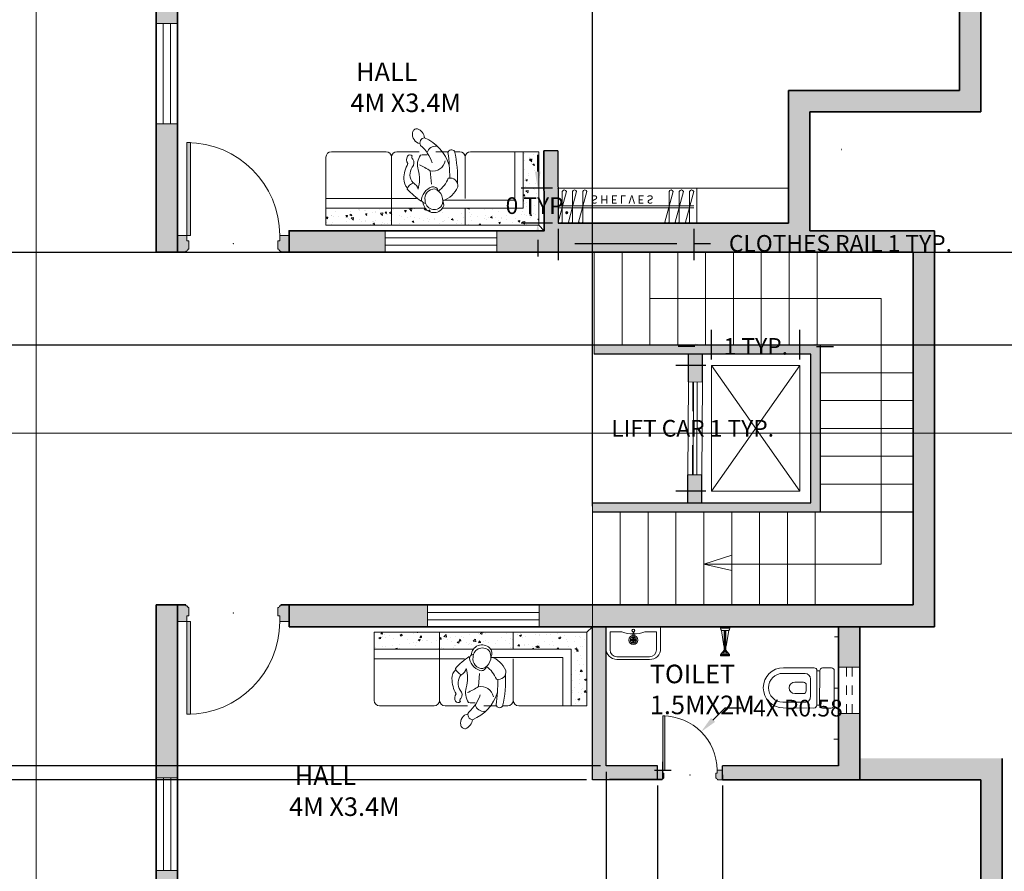
# Model space of a CAD drawing. Units: metres. Extents: x 2031 to 2061.8, y 1886.4 to 1909.8.
# Tile 8 of 10: x 2045.9 to 2056.5, y 1892.7 to 1901.9. Entities that reach past the tile are written whole.
import ezdxf

# ---------------------------------------------------------------- set-up
doc = ezdxf.new("R2010")
doc.units = ezdxf.units.M
doc.linetypes.add('DASHED', pattern=[0.75, 0.5, -0.25])
for name, color, linetype, lineweight in [('A-ANNO-DIMS', 2, 'Continuous', 18), ('A-ANNO-SYMB', 7, 'Continuous', 18), ('A-AREA-IDEN', 7, 'Continuous', 18), ('A-FLOR-CASE', 8, 'Continuous', 18), ('A-FLOR-EVTR', 4, 'Continuous', 18), ('A-FLOR-FIXT', 8, 'Continuous', 18), ('A-FLOR-STRS', 7, 'Continuous', 18), ('A-FLOR-STRS-PATH', 1, 'Continuous', 13), ('A-GLAZ-OVHD', 30, 'DASHED', 13), ('A-WALL-PATT', 252, 'Continuous', 13), ('doors & windows', 30, 'Continuous', 18), ('furniture', 24, 'Continuous', 13), ('inner walls', 4, 'Continuous', 25), ('windows', 30, 'Continuous', 18)]:
    doc.layers.add(name, color=color, linetype=linetype, lineweight=lineweight)
doc.layers.add('outer walls', color=1, linetype='Continuous', lineweight=35, plot=False)
doc.styles.get("Standard").update_dxf_attribs({"font": 'arial.ttf'})
doc.dimstyles.get("Standard").update_dxf_attribs({"dimtxt": 0.18, "dimasz": 0.18, "dimexe": 0.18, "dimexo": 0.0625, "dimgap": 0.09, "dimtad": 0, "dimtih": 1, "dimtoh": 1, "dimdec": 4, "dimzin": 0, "dimdsep": 46, "dimtxsty": 'Standard', "dimcen": 0.09, "dimadec": 0, "dimazin": 0, "dimtfac": 1, "dimtdec": 4, "dimtofl": 0, "dimtmove": 0, "dimatfit": 3, "dimfxl": 1, "dimtolj": 1, "dimtzin": 0, "dimarcsym": 0})

# ---------------------------------------------------------------- blocks, each defined once
blk = doc.blocks.new('D2')
at = {"layer": 'doors & windows'}
h = blk.add_hatch(dxfattribs=at)
h.set_pattern_fill('DOTS', color=256, scale=2, angle=180, style=0)
h.set_pattern_definition([(180, (0, -4), (-0.0625, -0.125), [0, -0.125])])
h.paths.add_polyline_path([(2.5, 0), (3.5, 0), (3.5, 24.98, 0.010003), (2.5, 25)])
h = blk.add_hatch(dxfattribs=at)
h.set_pattern_fill('DOTS', color=256, scale=2, angle=180, style=0)
h.set_pattern_definition([(180, (0, 0), (-0.0625, -0.125), [0, -0.125])])
edge = h.paths.add_edge_path()
edge.add_line((27.5, 0), (27.5, -1.5))
edge.add_line((27.5, -1.5), (27, -1.5))
edge.add_line((27, -1.5), (27, -3.75))
edge.add_line((27, -3.75), (27.25, -3.75))
edge.add_arc((27.76, -3.74), 0.509, 181.0059, 268.9941)
edge.add_line((27.75, -4.25), (27.75, -4.5))
edge.add_line((27.75, -4.5), (30, -4.5))
edge.add_line((30, -4.5), (30, 0))
edge.add_line((30, 0), (27.5, 0))
edge = h.paths.add_edge_path()
edge.add_line((2.5, -1.5), (2.5, 0))
edge.add_line((2.5, 0), (0, 0))
edge.add_line((0, 0), (0, -4.5))
edge.add_line((0, -4.5), (2.25, -4.5))
edge.add_line((2.25, -4.5), (2.25, -4.25))
edge.add_arc((2.24, -3.74), 0.509, 271.0059, 358.9941)
edge.add_line((2.75, -3.75), (3, -3.75))
edge.add_line((3, -3.75), (3, -1.5))
edge.add_line((3, -1.5), (2.5, -1.5))
for p, q in [((0, 0), (0, -4.5)), ((30, 0), (30, -4.5))]:
    blk.add_line(p, q)
blk.add_lwpolyline([(3.5, 0), (3.5, 25), (2.5, 25), (2.5, 0)], close=True, dxfattribs=at)
for points in [[(3, -3.75), (3, -1.5), (2.5, -1.5), (2.5, 0), (0, 0)], [(27, -3.75), (27, -1.5), (27.5, -1.5), (27.5, 0), (30, 0)], [(0, -4.5), (2.25, -4.5)], [(30, -4.5), (27.75, -4.5)]]:
    blk.add_lwpolyline(points, dxfattribs=at)
for points in [[(2.25, -4.5), (2.25, -4.25, 0.403966), (2.75, -3.75), (3, -3.75)], [(27.75, -4.5), (27.75, -4.25, -0.403966), (27.25, -3.75), (27, -3.75)]]:
    blk.add_lwpolyline(points, format="xyb", dxfattribs=at)
at = {"layer": 'doors & windows', "ltscale": 6}
blk.add_arc((2.5, 0), 25, 0, 90, dxfattribs=at)
at = {"layer": 'doors & windows'}
blk.add_point((15, -2.25), dxfattribs=at)
blk = doc.blocks.new('MAN')
at = {"layer": 'doors & windows'}
blk.add_line((1.3, -9.85), (0.89, -5.45), dxfattribs=at)
for centre, radius, start, end in [((0.1, 0.48), 3.6, 2.8928, 134.5528), ((-0.36, -7.56), 8.07, 108.0153, 157.5724), ((-0.81, 1.3), 2.37, 132.7993, 210.1219), ((1.3, 0.05), 4.16, 155.2349, 248.5051), ((0, 0), 3.06, 359.7942, 144.0351), ((-0.98, 0.55), 5.34, 289.2819, 356.6237), ((2.86, -0.44), 1.38, 352.7443, 87.7525), ((-8.99, -19.77), 24.04, 41.647, 56.3067), ((4.14, -10.82), 9.46, 125.6851, 158.6987), ((0.38, -2.75), 1.79, 192.3382, 283.0231), ((-0.1, -0.61), 3.22, 267.7788, 10.6507), ((-5.32, -4.92), 2.54, 170.002, 284.7527), ((34.75, -7.19), 42.53, 177.9613, 192.4551), ((15.87, -7.04), 10.97, 162.7002, 196.7262), ((8.59, -3.01), 3.29, 193.5598, 239.9446), ((5.83, -2.73), 3.32, 289.6374, 341.2911), ((3.84, -8.67), 4.24, 325.4363, 41.8446), ((6.12, -7.03), 4.01, 358.2671, 46.939), ((54.76, -7.35), 59.95, 180.1044, 188.2297), ((0.5, -14.05), 4.27, 79.2575, 168.509), ((-0.78, -6.94), 10.91, 330.7562, 358.8997), ((9.03, -7.36), 14.72, 197.1765, 246.7641), ((12.84, -8.62), 12.77, 197.9012, 229.3504), ((16.49, 13.41), 27.78, 236.8487, 245.427), ((-0.19, -11.81), 5.78, 325.2412, 16.1794), ((8.85, -12.54), 2.12, 136.0875, 215.1077), ((7.06, -13.61), 2.15, 328.4119, 38.6474), ((-5.78, -15.61), 1.25, 217.214, 345.0614), ((-0.4, -15.27), 2.81, 261.6005, 345.5998), ((3.21, -8.72), 6.53, 262.8142, 281.931), ((6.8, -14.37), 0.689, 315.9836, 61.7947), ((8.05, -14.12), 1.05, 224.0636, 323.687), ((3.09, -19.2), 1.68, 274.444, 31.8659), ((4.09, -22.01), 3.16, 349.15, 77.9716), ((6.99, -20.36), 3.8, 187.9766, 248.0432), ((5.75, -22.44), 1.45, 262.6631, 353.5986)]:
    blk.add_arc(centre, radius, start, end, dxfattribs=at)
blk = doc.blocks.new('sofa 2')
at = {"layer": 'furniture', "ltscale": 0.5}
h = blk.add_hatch(dxfattribs=at)
h.set_pattern_fill('AR-CONC', color=256, angle=450, style=0)
h.set_pattern_definition([(40, (-1099.1507, 871.655), (-0.627521, 7.172602), [0.75, -8.25]), (95, (-1099.151, 871.655), (7.52192, -1.387513), [0.6, -6.6]), (349.5486, (-1099.203, 872.253), (6.894395, 5.785094), [0.637402, -7.01142]), (43.8158, (-1097.151, 871.655), (-1.65519, 10.67241), [1.125, -12.375]), (353.3644, (-1097.289, 872.544), (9.74118, 9.34663), [0.9561, -10.51713]), (98.8158, (-1097.151, 871.655), (9.74119, 9.34662), [0.9, -9.9]), (69, (-1097.6507, 872.655), (-4.02619, 5.96907), [0.75, -8.25]), (124, (-1097.651, 872.655), (7.2515, 2.433153), [0.6, -6.6]), (18.5486, (-1097.986, 873.1524), (3.225305, 8.402226), [0.637402, -7.01142]), (52.5, (-1099.1507, 871.655), (3.3289385, 0.1215986), [0, -6.52, 0, -6.7, 0, -6.625]), (82.5, (-1099.1507, 871.655), (3.944117, 2.630695), [0, -3.82, 0, -6.37, 0, -2.525]), (122.5, (-1099.1507, 869.425), (-0.2255487, 5.3382244), [0, -2.5, 0, -7.8, 0, -10.35]), (132.5, (-1099.1507, 868.425), (1.00105, 5.831862), [0, -3.25, 0, -5.18, 0, -7.35])])
h.paths.add_polyline_path([(-8.27, -37.7, 0.168872), (-7.9, -36.76, 0.613808), (-6.95, -30.77, 0.074869), (-8.27, -30.38), (-8.27, -29), (-2, -29), (-2, -56), (-8.27, -56)])
h.paths.add_polyline_path([(-8.27, -7.77), (-29, -7.77), (-29, -2), (-2, -2), (-2, -29), (-8.27, -29)])
h.paths.add_polyline_path([(-8.27, -80), (-2, -80), (-2, -56), (-8.27, -56)])
at = {"layer": 'furniture'}
for p, q in [((-2, -2), (0, 0)), ((-29, -2), (-2, -2)), ((-29, -27), (-29, -2)), ((-2, -2), (-2, -80)), ((-8.27, -7.77), (-29, -7.77)), ((-11.27, -10.77), (-29, -10.77)), ((-11.27, -37.27), (-11.27, -10.77)), ((-8.27, -37.27), (-8.27, -7.77)), ((-29, -32.87), (-29, -31)), ((-27, -29), (-11.8, -29)), ((-8.27, -29), (-2, -29)), ((-29, -39.74), (-29, -35.16)), ((-8.27, -37.7), (-8.27, -37.7)), ((-29, -45.8), (-29, -54)), ((-11.8, -80), (-11.8, -46.89)), ((-8.27, -43.66), (-8.27, -80)), ((-27, -56), (-2, -56)), ((-29, -78), (-29, -58)), ((-2, -80), (-27, -80))]:
    blk.add_line(p, q, dxfattribs=at)
for centre, start, end in [((-27, -27), 180, 270), ((-27, -31), 90, 180), ((-27, -54), 180, 270), ((-27, -58), 90, 180), ((-27, -78), 180, 270)]:
    blk.add_arc(centre, 2, start, end, dxfattribs=at)
at = {"xscale": 1.099999999999999, "yscale": 1.099999999999999, "zscale": 1.099999999999999, "rotation": 270}
blk.add_blockref('MAN', (-11.13, -40.34), dxfattribs=at)
blk = doc.blocks.new('hangers')
at = {"layer": 'furniture'}
for p, q in [((0, 16.5), (4, 1.5)), ((2, 16.5), (2, 1.5)), ((5, 16.5), (9, 1.5)), ((7, 16.5), (7, 1.5)), ((10, 16.5), (14, 1.5)), ((12, 16.5), (12, 1.5)), ((52, 16.5), (56, 1.5)), ((54, 16.5), (54, 1.5)), ((57, 16.5), (61, 1.5)), ((59, 16.5), (59, 1.5)), ((62, 16.5), (66, 1.5)), ((64, 16.5), (64, 1.5)), ((66, 9.5), (0, 9.5)), ((0, 8.5), (66, 8.5))]:
    blk.add_line(p, q, dxfattribs=at)
for centre, radius, start, end in [((1, 15.62), 1.33, 41.2884, 138.7116), ((6, 15.62), 1.33, 41.2884, 138.7116), ((11, 15.62), 1.33, 41.2884, 138.7116), ((53, 15.62), 1.33, 41.2884, 138.7116), ((58, 15.62), 1.33, 41.2884, 138.7116), ((63, 15.62), 1.33, 41.2884, 138.7116), ((3, 1.92), 1.08, 202.5549, 337.4451), ((8, 1.92), 1.08, 202.5549, 337.4451), ((13, 1.92), 1.08, 202.5549, 337.4451), ((55, 1.92), 1.08, 202.5549, 337.4451), ((60, 1.92), 1.08, 202.5549, 337.4451), ((65, 1.92), 1.08, 202.5549, 337.4451)]:
    blk.add_arc(centre, radius, start, end, dxfattribs=at)
blk.add_point((0, 0), dxfattribs=at)
blk.add_text('S H E L V E S', height=4, dxfattribs=at).set_placement((16, 3.48))
blk = doc.blocks.new('commode')
for p, q in [((-7.09, 19.41), (-7.09, 8.61)), ((-5.09, 11.81), (-5.09, 19.57)), ((5.09, 11.81), (5.09, 19.57)), ((7.09, 19.41), (7.09, 8.61)), ((-2, 12.37), (-2, 15.37)), ((2, 12.37), (2, 15.37)), ((-1, 11.37), (1, 11.37)), ((-6.09, 7.61), (6.09, 7.61)), ((-6.09, 6.61), (-6.09, 7.61)), ((-3.15, 9.87), (3.15, 9.87)), ((6.09, 7.61), (6.09, 6.61)), ((-7.09, 2.5), (-7.09, 5.61)), ((-6.09, 6.61), (6.09, 6.61)), ((7.09, 2.5), (7.09, 5.61)), ((-18, 1.5), (-18, 0)), ((-6.09, 1.5), (6.09, 1.5)), ((0, 1.5), (0, 0)), ((18, 1.5), (18, 0))]:
    blk.add_line(p, q)
for centre, radius, start, end in [((0, 19.41), 7.09, 0, 180), ((0, 19.57), 5.09, 0, 180), ((0, 15.37), 2, 0, 180), ((-3.15, 11.81), 1.94, 180, 270), ((-1, 12.37), 1, 180, 270), ((1, 12.37), 1, 270, 0), ((3.15, 11.81), 1.94, 270, 0), ((-6.09, 8.61), 1, 180, 270), ((6.09, 8.61), 1, 270, 0), ((-6.09, 5.61), 1, 90, 180), ((6.09, 5.61), 1, 0, 90), ((-6.09, 2.5), 1, 180, 270), ((6.09, 2.5), 1, 270, 0)]:
    blk.add_arc(centre, radius, start, end)
blk = doc.blocks.new('wash basin 1')
for p, q in [((-8.5, 8.5), (-1.85, 8.5)), ((0, 10), (-8, 10)), ((-1.85, 8.5), (-1.85, 4.19)), ((0, 10), (0, -10)), ((-12, 6), (-12, -6)), ((-11, 6), (-11, -6)), ((-1.85, -8.5), (-1.85, -4.19)), ((-8.5, -8.5), (-1.85, -8.5)), ((0, -10), (-8, -10))]:
    blk.add_line(p, q)
blk.add_lwpolyline([(-1.83, 0.11), (-5.25, 0.25), (-5.23, -0.38), (-1.8, -0.19)])
for centre, radius in [((-4.87, 0), 1.68), ((-4.87, 0), 1.18), ((-5.63, 0), 0.25), ((-4.87, 0.75), 0.25), ((-4.87, 0), 0.25), ((-4.19, 0), 0.25), ((-1.34, 0), 0.5), ((-4.87, -0.72), 0.25)]:
    blk.add_circle(centre, radius)
for centre, radius, start, end in [((-8, 6), 4, 90, 180), ((-8.5, 6), 2.5, 90, 180), ((8.89, 0), 11.53, 158.7059, 201.2941), ((-8, -6), 4, 180, 270), ((-8.5, -6), 2.5, 180, 270)]:
    blk.add_arc(centre, radius, start, end)
blk = doc.blocks.new('tap & shower')
for p, q in [((1.71, 0), (-1.71, 0)), ((-1.71, 0), (-1.71, -0.5)), ((1.71, 0), (1.71, -0.5)), ((1.71, -0.5), (-1.71, -0.5)), ((1.31, -1.4), (-1.31, -1.4)), ((-1.31, -1.4), (-0.39, -7)), ((-0.32, -0.5), (0.32, -0.5)), ((-0.27, -7.94), (-0.27, -1.4)), ((-0.22, -7.94), (-0.22, -1.4)), ((-0.16, -7.94), (-0.16, -1.4)), ((0, -8.48), (0, -1.4)), ((0.16, -7.94), (0.16, -1.4)), ((0.22, -7.94), (0.22, -1.4)), ((0.27, -7.94), (0.27, -1.4)), ((0.39, -7), (1.31, -1.4)), ((-1.62, -10.37), (-1.62, -10.1)), ((-1.48, -9.96), (-0.27, -8.48)), ((-1.48, -9.96), (1.48, -9.96)), ((-1.48, -10.5), (-1.48, -9.96)), ((-1.48, -10.5), (1.48, -10.5)), ((-1.43, -10.5), (-1.43, -9.96)), ((-1.37, -10.5), (-1.37, -9.96)), ((-1.32, -10.5), (-1.32, -9.96)), ((-1.27, -10.5), (-1.27, -9.96)), ((-1.21, -10.5), (-1.21, -9.96)), ((-1.16, -10.5), (-1.16, -9.96)), ((-1.1, -10.5), (-1.1, -9.96)), ((-1.05, -10.5), (-1.05, -9.96)), ((-1, -10.5), (-1, -9.96)), ((-0.21, -8.48), (-0.94, -9.96)), ((-0.94, -10.5), (-0.94, -9.96)), ((-0.89, -10.5), (-0.89, -9.96)), ((-0.84, -10.5), (-0.84, -9.96)), ((-0.78, -10.5), (-0.78, -9.96)), ((-0.73, -10.5), (-0.73, -9.96)), ((-0.67, -10.5), (-0.67, -9.96)), ((-0.62, -10.5), (-0.62, -9.96)), ((-0.57, -10.5), (-0.57, -9.96)), ((-0.51, -10.5), (-0.51, -9.96)), ((-0.46, -10.5), (-0.46, -9.96)), ((-0.09, -8.48), (-0.4, -9.96)), ((-0.4, -10.5), (-0.4, -9.96)), ((-0.35, -10.5), (-0.35, -9.96)), ((-0.32, -7.94), (0.32, -7.94)), ((-0.32, -8.48), (-0.32, -7.94)), ((-0.32, -8.48), (0.32, -8.48)), ((-0.3, -10.5), (-0.3, -9.96)), ((-0.24, -10.5), (-0.24, -9.96)), ((-0.19, -10.5), (-0.19, -9.96)), ((-0.13, -10.5), (-0.13, -9.96)), ((-0.08, -10.5), (-0.08, -9.96)), ((-0.03, -10.5), (-0.03, -9.96)), ((0.03, -10.5), (0.03, -9.96)), ((0.08, -10.5), (0.08, -9.96)), ((0.09, -8.48), (0.4, -9.96)), ((0.13, -10.5), (0.13, -9.96)), ((0.19, -10.5), (0.19, -9.96)), ((0.21, -8.48), (0.94, -9.96)), ((0.24, -10.5), (0.24, -9.96)), ((1.48, -9.96), (0.27, -8.48)), ((0.3, -10.5), (0.3, -9.96)), ((0.32, -8.48), (0.32, -7.94)), ((0.35, -10.5), (0.35, -9.96)), ((0.4, -10.5), (0.4, -9.96)), ((0.46, -10.5), (0.46, -9.96)), ((0.51, -10.5), (0.51, -9.96)), ((0.57, -10.5), (0.57, -9.96)), ((0.62, -10.5), (0.62, -9.96)), ((0.67, -10.5), (0.67, -9.96)), ((0.73, -10.5), (0.73, -9.96)), ((0.78, -10.5), (0.78, -9.96)), ((0.84, -10.5), (0.84, -9.96)), ((0.89, -10.5), (0.89, -9.96)), ((0.94, -10.5), (0.94, -9.96)), ((1, -10.5), (1, -9.96)), ((1.05, -10.5), (1.05, -9.96)), ((1.1, -10.5), (1.1, -9.96)), ((1.16, -10.5), (1.16, -9.96)), ((1.21, -10.5), (1.21, -9.96)), ((1.27, -10.5), (1.27, -9.96)), ((1.32, -10.5), (1.32, -9.96)), ((1.37, -10.5), (1.37, -9.96)), ((1.43, -10.5), (1.43, -9.96)), ((1.48, -10.5), (1.48, -9.96)), ((1.62, -10.37), (1.62, -10.1))]:
    blk.add_line(p, q)
for centre, radius, start, end in [((-0.02, -0.29), 1.7, 187.1825, 220.9028), ((0.02, -0.29), 1.7, 319.0972, 352.8175), ((0, -6.99), 0.392, 181.7992, 358.2008), ((-1.48, -10.1), 0.135, 90, 180), ((-1.48, -10.37), 0.135, 180, 270), ((1.48, -10.1), 0.135, 0, 90), ((1.48, -10.37), 0.135, 270, 0)]:
    blk.add_arc(centre, radius, start, end)
blk = doc.blocks.new('WIN-1200')
for p, q in [((0.23, 1.2), (0, 1.2)), ((0.075, 0), (0.075, 1.2)), ((0.155, 0), (0.155, 1.2)), ((0.23, 0), (0, 0))]:
    blk.add_line(p, q)
blk = doc.blocks.new('LIFT-CAR-PLAN')
for p, q in [((0.951, 0), (0, 1.357)), ((0, 0), (0.951, 1.357))]:
    blk.add_line(p, q)
blk.add_lwpolyline([(0, 1.357), (0.951, 1.357), (0.951, 0), (0, 0)], close=True)
blk = doc.blocks.new('*D38')
at = {"layer": 'A-ANNO-DIMS', "color": 0, "lineweight": -2, "transparency": 16777216}
for p, q in [((2051.671, 1899.622), (2051.671, 1899.285)), ((2053.131, 1899.622), (2053.131, 1899.285)), ((2051.851, 1899.465), (2052.951, 1899.465)), ((2053.131, 1899.465), (2053.311, 1899.465))]:
    blk.add_line(p, q, dxfattribs=at)
at = {"layer": 'A-ANNO-DIMS', "color": 0, "transparency": 16777216}
for points in [[(2051.851, 1899.495), (2051.851, 1899.435), (2051.671, 1899.465)], [(2052.951, 1899.495), (2052.951, 1899.435), (2053.131, 1899.465)]]:
    blk.add_solid(points, dxfattribs=at)
at = {"layer": 'Defpoints', "color": 0, "transparency": 16777216}
for p in [(2051.671, 1899.684), (2053.131, 1899.684), (2053.131, 1899.465)]:
    blk.add_point(p, dxfattribs=at)
at = {"layer": 'A-ANNO-DIMS', "color": 0, "transparency": 16777216, "insert": (2054.711, 1899.465), "char_height": 0.18, "attachment_point": 5}
blk.add_mtext('\\A1;CLOTHES RAIL 1 TYP.', dxfattribs=at)
blk = doc.blocks.new('*D39')
at = {"layer": 'A-ANNO-DIMS', "color": 0, "lineweight": -2, "transparency": 16777216}
for p, q in [((2051.452, 1900.239), (2051.452, 1900.419)), ((2051.609, 1900.059), (2051.272, 1900.059)), ((2051.609, 1899.684), (2051.272, 1899.684)), ((2051.452, 1899.504), (2051.452, 1899.324))]:
    blk.add_line(p, q, dxfattribs=at)
at = {"layer": 'A-ANNO-DIMS', "color": 0, "transparency": 16777216}
for points in [[(2051.422, 1900.239), (2051.482, 1900.239), (2051.452, 1900.059)], [(2051.422, 1899.504), (2051.482, 1899.504), (2051.452, 1899.684)]]:
    blk.add_solid(points, dxfattribs=at)
at = {"layer": 'Defpoints', "color": 0, "transparency": 16777216}
for p in [(2051.671, 1900.059), (2051.452, 1899.684), (2051.671, 1899.684)]:
    blk.add_point(p, dxfattribs=at)
at = {"layer": 'A-ANNO-DIMS', "color": 0, "transparency": 16777216, "insert": (2051.452, 1899.872), "char_height": 0.18, "attachment_point": 5}
blk.add_mtext('\\A1;0 TYP.', dxfattribs=at)
blk = doc.blocks.new('*D42')
at = {"layer": 'A-ANNO-DIMS', "color": 0, "lineweight": -2, "transparency": 16777216}
for p, q in [((2053.262, 1898.151), (2052.94, 1898.151)), ((2053.12, 1897.971), (2053.12, 1897.656)), ((2053.12, 1896.974), (2053.12, 1897.29)), ((2053.262, 1896.794), (2052.94, 1896.794))]:
    blk.add_line(p, q, dxfattribs=at)
at = {"layer": 'A-ANNO-DIMS', "color": 0, "transparency": 16777216}
for points in [[(2053.09, 1897.971), (2053.15, 1897.971), (2053.12, 1898.151)], [(2053.09, 1896.974), (2053.15, 1896.974), (2053.12, 1896.794)]]:
    blk.add_solid(points, dxfattribs=at)
at = {"layer": 'Defpoints', "color": 0, "transparency": 16777216}
for p in [(2053.12, 1898.151), (2053.324, 1898.151), (2053.324, 1896.794)]:
    blk.add_point(p, dxfattribs=at)
at = {"layer": 'A-ANNO-DIMS', "color": 0, "transparency": 16777216, "insert": (2053.12, 1897.473), "char_height": 0.18, "attachment_point": 5}
blk.add_mtext('\\A1;LIFT CAR 1 TYP.', dxfattribs=at)
blk = doc.blocks.new('*D43')
at = {"layer": 'A-ANNO-DIMS', "color": 0, "lineweight": -2, "transparency": 16777216}
for p, q in [((2053.324, 1898.214), (2053.324, 1898.535)), ((2054.275, 1898.214), (2054.275, 1898.535)), ((2053.144, 1898.355), (2052.964, 1898.355)), ((2054.455, 1898.355), (2054.635, 1898.355))]:
    blk.add_line(p, q, dxfattribs=at)
at = {"layer": 'A-ANNO-DIMS', "color": 0, "transparency": 16777216}
for points in [[(2053.144, 1898.385), (2053.144, 1898.325), (2053.324, 1898.355)], [(2054.455, 1898.385), (2054.455, 1898.325), (2054.275, 1898.355)]]:
    blk.add_solid(points, dxfattribs=at)
at = {"layer": 'Defpoints', "color": 0, "transparency": 16777216}
for p in [(2054.275, 1898.355), (2053.324, 1898.151), (2054.275, 1898.151)]:
    blk.add_point(p, dxfattribs=at)
at = {"layer": 'A-ANNO-DIMS', "color": 0, "transparency": 16777216, "insert": (2053.8, 1898.355), "char_height": 0.18, "attachment_point": 5}
blk.add_mtext('\\A1;1 TYP.', dxfattribs=at)
blk = doc.blocks.new('*D44')
at = {"layer": 'A-ANNO-DIMS', "color": 0, "lineweight": -2, "transparency": 16777216}
for p, q in [((2036.233, 1900.72), (2036.233, 1886.39)), ((2056.454, 1889.993), (2056.454, 1886.39)), ((2036.413, 1886.57), (2045.949, 1886.57)), ((2056.274, 1886.57), (2046.738, 1886.57))]:
    blk.add_line(p, q, dxfattribs=at)
at = {"layer": 'A-ANNO-DIMS', "color": 0, "transparency": 16777216}
for points in [[(2036.413, 1886.6), (2036.413, 1886.54), (2036.233, 1886.57)], [(2056.274, 1886.6), (2056.274, 1886.54), (2056.454, 1886.57)]]:
    blk.add_solid(points, dxfattribs=at)
at = {"layer": 'Defpoints', "color": 0, "transparency": 16777216}
for p in [(2036.233, 1900.782), (2056.454, 1890.056), (2056.454, 1886.57)]:
    blk.add_point(p, dxfattribs=at)
at = {"layer": 'A-ANNO-DIMS', "color": 0, "transparency": 16777216, "insert": (2046.343, 1886.57), "char_height": 0.18, "attachment_point": 5}
blk.add_mtext('\\A1;20.22', dxfattribs=at)
blk = doc.blocks.new('*D45')
at = {"layer": 'A-ANNO-DIMS', "color": 0, "lineweight": -2, "transparency": 16777216}
for p, q in [((2047.556, 1907.081), (2061.614, 1907.081)), ((2061.434, 1906.901), (2061.434, 1897.862)), ((2061.434, 1888.459), (2061.434, 1897.498)), ((2054.286, 1888.279), (2061.614, 1888.279))]:
    blk.add_line(p, q, dxfattribs=at)
at = {"layer": 'A-ANNO-DIMS', "color": 0, "transparency": 16777216}
for points in [[(2061.404, 1906.901), (2061.464, 1906.901), (2061.434, 1907.081)], [(2061.404, 1888.459), (2061.464, 1888.459), (2061.434, 1888.279)]]:
    blk.add_solid(points, dxfattribs=at)
at = {"layer": 'Defpoints', "color": 0, "transparency": 16777216}
for p in [(2047.494, 1907.081), (2061.434, 1907.081), (2054.224, 1888.279)]:
    blk.add_point(p, dxfattribs=at)
at = {"layer": 'A-ANNO-DIMS', "color": 0, "transparency": 16777216, "insert": (2061.434, 1897.68), "char_height": 0.18, "attachment_point": 5}
blk.add_mtext('\\A1;18.802', dxfattribs=at)
blk = doc.blocks.new('*D57')
at = {"layer": 'A-ANNO-DIMS', "color": 0, "lineweight": -2, "transparency": 16777216}
for p, q in [((2040.478, 1899.371), (2061.614, 1899.371)), ((2061.434, 1899.191), (2061.434, 1899.052)), ((2061.434, 1898.551), (2061.434, 1898.691)), ((2040.478, 1898.371), (2061.614, 1898.371))]:
    blk.add_line(p, q, dxfattribs=at)
at = {"layer": 'A-ANNO-DIMS', "color": 0, "transparency": 16777216}
for points in [[(2061.404, 1899.191), (2061.464, 1899.191), (2061.434, 1899.371)], [(2061.404, 1898.551), (2061.464, 1898.551), (2061.434, 1898.371)]]:
    blk.add_solid(points, dxfattribs=at)
at = {"layer": 'Defpoints', "color": 0, "transparency": 16777216}
for p in [(2040.416, 1899.371), (2061.434, 1899.371), (2040.416, 1898.371)]:
    blk.add_point(p, dxfattribs=at)
at = {"layer": 'A-ANNO-DIMS', "color": 0, "transparency": 16777216, "insert": (2061.434, 1898.871), "char_height": 0.18, "attachment_point": 5}
blk.add_mtext('\\A1;1', dxfattribs=at)
blk = doc.blocks.new('*D58')
at = {"layer": 'A-ANNO-DIMS', "color": 0, "lineweight": -2, "transparency": 16777216}
for p, q in [((2040.416, 1896.634), (2040.416, 1909.841)), ((2052.04, 1896.634), (2052.04, 1909.841)), ((2040.596, 1909.661), (2045.773, 1909.661)), ((2051.86, 1909.661), (2046.683, 1909.661))]:
    blk.add_line(p, q, dxfattribs=at)
at = {"layer": 'A-ANNO-DIMS', "color": 0, "transparency": 16777216}
for points in [[(2040.596, 1909.691), (2040.596, 1909.631), (2040.416, 1909.661)], [(2051.86, 1909.691), (2051.86, 1909.631), (2052.04, 1909.661)]]:
    blk.add_solid(points, dxfattribs=at)
at = {"layer": 'Defpoints', "color": 0, "transparency": 16777216}
for p in [(2052.04, 1909.661), (2040.416, 1896.571), (2052.04, 1896.571)]:
    blk.add_point(p, dxfattribs=at)
at = {"layer": 'A-ANNO-DIMS', "color": 0, "transparency": 16777216, "insert": (2046.228, 1909.661), "char_height": 0.18, "attachment_point": 5}
blk.add_mtext('\\A1;11.624', dxfattribs=at)
blk = doc.blocks.new('*D61')
at = {"layer": 'A-ANNO-DIMS', "color": 0, "lineweight": -2, "transparency": 16777216}
for p, q in [((2031.745, 1894.015), (2031.745, 1894.195)), ((2031.745, 1894.195), (2031.925, 1894.195)), ((2052.128, 1893.835), (2031.565, 1893.835)), ((2051.978, 1893.685), (2031.565, 1893.685)), ((2031.745, 1893.505), (2031.745, 1893.325))]:
    blk.add_line(p, q, dxfattribs=at)
at = {"layer": 'A-ANNO-DIMS', "color": 0, "transparency": 16777216}
for points in [[(2031.715, 1894.015), (2031.775, 1894.015), (2031.745, 1893.835)], [(2031.715, 1893.505), (2031.775, 1893.505), (2031.745, 1893.685)]]:
    blk.add_solid(points, dxfattribs=at)
at = {"layer": 'Defpoints', "color": 0, "transparency": 16777216}
for p in [(2031.745, 1893.835), (2052.19, 1893.835), (2052.04, 1893.685)]:
    blk.add_point(p, dxfattribs=at)
at = {"layer": 'A-ANNO-DIMS', "color": 0, "transparency": 16777216, "insert": (2032.249, 1894.195), "char_height": 0.18, "attachment_point": 5}
blk.add_mtext('\\A1;0.15', dxfattribs=at)
blk = doc.blocks.new('*D62')
at = {"layer": 'A-ANNO-DIMS', "color": 0, "lineweight": -2, "transparency": 16777216}
for p, q in [((2052.19, 1893.772), (2052.19, 1886.39)), ((2052.74, 1893.623), (2052.74, 1886.39)), ((2052.37, 1886.57), (2052.56, 1886.57)), ((2052.74, 1886.57), (2052.92, 1886.57))]:
    blk.add_line(p, q, dxfattribs=at)
at = {"layer": 'A-ANNO-DIMS', "color": 0, "transparency": 16777216}
for points in [[(2052.37, 1886.6), (2052.37, 1886.54), (2052.19, 1886.57)], [(2052.56, 1886.6), (2052.56, 1886.54), (2052.74, 1886.57)]]:
    blk.add_solid(points, dxfattribs=at)
at = {"layer": 'Defpoints', "color": 0, "transparency": 16777216}
for p in [(2052.19, 1893.835), (2052.74, 1893.686), (2052.74, 1886.57)]:
    blk.add_point(p, dxfattribs=at)
at = {"layer": 'A-ANNO-DIMS', "color": 0, "transparency": 16777216, "insert": (2053.245, 1886.57), "char_height": 0.18, "attachment_point": 5}
blk.add_mtext('\\A1;0.55', dxfattribs=at)
blk = doc.blocks.new('*D63')
at = {"layer": 'A-ANNO-DIMS', "color": 0, "lineweight": -2, "transparency": 16777216}
for p, q in [((2052.74, 1893.623), (2052.74, 1886.39)), ((2053.44, 1893.624), (2053.44, 1886.39)), ((2052.92, 1886.57), (2053.26, 1886.57)), ((2053.44, 1886.57), (2053.62, 1886.57))]:
    blk.add_line(p, q, dxfattribs=at)
at = {"layer": 'A-ANNO-DIMS', "color": 0, "transparency": 16777216}
for points in [[(2052.92, 1886.6), (2052.92, 1886.54), (2052.74, 1886.57)], [(2053.26, 1886.6), (2053.26, 1886.54), (2053.44, 1886.57)]]:
    blk.add_solid(points, dxfattribs=at)
at = {"layer": 'Defpoints', "color": 0, "transparency": 16777216}
for p in [(2052.74, 1893.686), (2053.44, 1893.686), (2053.44, 1886.57)]:
    blk.add_point(p, dxfattribs=at)
at = {"layer": 'A-ANNO-DIMS', "color": 0, "transparency": 16777216, "insert": (2053.874, 1886.57), "char_height": 0.18, "attachment_point": 5}
blk.add_mtext('\\A1;0.7', dxfattribs=at)
blk = doc.blocks.new('*D66')
at = {"layer": 'A-ANNO-DIMS', "color": 0, "lineweight": -2, "transparency": 16777216}
for p, q in [((2053.466, 1894.458), (2053.338, 1894.33)), ((2053.646, 1894.458), (2053.466, 1894.458)), ((2052.709, 1893.791), (2052.889, 1893.791)), ((2052.799, 1893.701), (2052.799, 1893.881))]:
    blk.add_line(p, q, dxfattribs=at)
at = {"layer": 'A-ANNO-DIMS', "color": 0, "transparency": 16777216}
blk.add_solid([(2053.317, 1894.352), (2053.36, 1894.309), (2053.211, 1894.203)], dxfattribs=at)
at = {"layer": 'Defpoints', "color": 0, "transparency": 16777216}
for p in [(2053.211, 1894.203), (2052.799, 1893.791)]:
    blk.add_point(p, dxfattribs=at)
at = {"layer": 'A-ANNO-DIMS', "color": 0, "transparency": 16777216, "insert": (2054.253, 1894.458), "char_height": 0.18, "attachment_point": 5}
blk.add_mtext('\\A1;4X R0.58', dxfattribs=at)

msp = doc.modelspace()

# ---------------------------------------------------------------- hatches: boundary and pattern name
at = {"layer": 'A-WALL-PATT'}
h = msp.add_hatch(color=256, dxfattribs=at)
h.dxf.hatch_style = 1
h.paths.add_polyline_path([(2055.7239, 1899.6012), (2054.3827, 1899.6012), (2054.3827, 1900.8841), (2056.2239, 1900.8841), (2056.2239, 1902.2385), (2055.9939, 1902.2385), (2055.9939, 1901.1141), (2054.1527, 1901.1141), (2054.1527, 1899.6841), (2051.6718, 1899.6841), (2051.6687, 1900.4631), (2051.5187, 1900.4625), (2051.5221, 1899.6012), (2051.0102, 1899.6012), (2051.0102, 1899.3712), (2054.7239, 1899.3712), (2055.4939, 1899.3712), (2055.4939, 1895.5712), (2052.04, 1895.5712), (2052.04, 1895.3348), (2055.7239, 1895.3348)])
h.paths.add_polyline_path([(2056.2239, 1904.7441), (2054.3039, 1904.7441), (2054.3039, 1906.3941), (2054.1539, 1906.3941), (2054.1539, 1904.7441), (2052.3539, 1904.7441), (2052.3539, 1904.5141), (2055.9939, 1904.5141), (2055.9939, 1903.4385), (2056.2239, 1903.4385)])
h.paths.add_polyline_path([(2051.6539, 1906.3941), (2051.5039, 1906.3941), (2051.5039, 1904.7441), (2051.0735, 1904.7441), (2051.0735, 1904.5141), (2051.5039, 1904.5141), (2051.5039, 1903.2141), (2051.6539, 1903.2141), (2051.6539, 1904.5141), (2051.6539, 1904.7441)])
h.paths.add_polyline_path([(2050.5735, 1904.7441), (2049.2597, 1904.7441), (2049.2597, 1904.5141), (2049.8539, 1904.5141), (2049.8539, 1902.3641), (2051.6572, 1902.3641), (2051.6567, 1902.5141), (2051.5489, 1902.5141), (2050.0039, 1902.5141), (2050.0039, 1903.1021), (2050.0039, 1904.5141), (2050.5735, 1904.5141)])
h.paths.add_polyline_path([(2048.2597, 1904.7441), (2047.4939, 1904.7441), (2047.4939, 1907.0812), (2047.3439, 1907.0812), (2047.3439, 1901.8355), (2047.5739, 1901.8355), (2047.5739, 1902.1341), (2048.0857, 1902.1341), (2048.0857, 1902.2841), (2047.5739, 1902.2841), (2047.5739, 1904.5141), (2048.2597, 1904.5141)])
h.paths.add_polyline_path([(2047.5739, 1900.7526), (2047.3439, 1900.7526), (2047.3439, 1899.3712), (2047.5739, 1899.3712), (2047.5739, 1899.5512)])
h.paths.add_polyline_path([(2049.8102, 1899.6012), (2048.7739, 1899.6012), (2048.7739, 1899.3712), (2049.8102, 1899.3712)])
h = msp.add_hatch(color=256, dxfattribs=at)
h.dxf.hatch_style = 1
h.paths.add_polyline_path([(2055.7239, 1895.3348), (2055.7239, 1899.6012), (2054.7239, 1899.6012), (2054.7239, 1899.3712), (2055.4939, 1899.3712), (2055.4939, 1895.5712), (2052.04, 1895.5712), (2052.04, 1895.3348)])
h = msp.add_hatch(color=256, dxfattribs=at)
h.dxf.hatch_style = 1
h.paths.add_polyline_path([(2053.2265, 1898.2712), (2053.0765, 1898.2712), (2053.0747, 1897.9721), (2053.2247, 1897.9712)], flags=17)
h.paths.add_polyline_path([(2052.059, 1898.3712), (2052.059, 1898.2712), (2054.3939, 1898.2712), (2054.3939, 1896.6712), (2052.04, 1896.6712), (2052.04, 1896.5712), (2054.4939, 1896.5712), (2054.4939, 1898.3712)])
h = msp.add_hatch(color=256, dxfattribs=at)
h.dxf.hatch_style = 1
h.paths.add_polyline_path([(2053.2187, 1896.9712), (2053.0687, 1896.9721), (2053.067, 1896.6712), (2053.217, 1896.6712)])
h = msp.add_hatch(color=256, dxfattribs=at)
h.dxf.hatch_style = 1
h.paths.add_polyline_path([(2051.5739, 1890.0556), (2051.4239, 1890.0556), (2051.4239, 1889.8182), (2049.7239, 1889.8182), (2049.7239, 1891.8184), (2050.3473, 1891.8184), (2050.3473, 1891.9684), (2049.5739, 1891.9684), (2049.5739, 1889.8182), (2049.2545, 1889.8182), (2049.2545, 1889.5882), (2051.4239, 1889.5882), (2051.4239, 1888.279), (2051.5739, 1888.279)])
h.paths.add_polyline_path([(2048.5112, 1889.8182), (2047.5739, 1889.8182), (2047.5739, 1891.8184), (2048.0857, 1891.8184), (2048.0857, 1891.9684), (2047.5739, 1891.9684), (2047.5739, 1892.708), (2047.3439, 1892.708), (2047.3439, 1889.5882), (2048.5112, 1889.5882)])
h.paths.add_polyline_path([(2047.5739, 1895.3348), (2047.5739, 1895.5712), (2047.3439, 1895.5712), (2047.3439, 1893.708), (2047.5739, 1893.708)])
h = msp.add_hatch(color=256, dxfattribs=at)
h.dxf.hatch_style = 1
h.paths.add_polyline_path([(2050.2655, 1895.5712), (2048.7739, 1895.5712), (2048.7739, 1895.3348), (2050.2655, 1895.3348)])
h.paths.add_polyline_path([(2052.04, 1895.5712), (2051.4655, 1895.5712), (2051.4655, 1895.3348), (2052.04, 1895.3348)])
h = msp.add_hatch(color=256, dxfattribs=at)
h.dxf.hatch_style = 1
h.paths.add_polyline_path([(2054.92, 1894.4001), (2054.69, 1894.4001), (2054.69, 1893.8348), (2053.4402, 1893.8348), (2053.4402, 1893.6864), (2054.92, 1893.688)])
h.paths.add_polyline_path([(2054.92, 1895.3348), (2054.69, 1895.3348), (2054.69, 1894.9001), (2054.92, 1894.9001)])
h.paths.add_polyline_path([(2052.19, 1895.071, -0.0627034), (2052.1864, 1895.1002), (2052.1869, 1895.3348), (2052.04, 1895.3348), (2052.04, 1893.6848), (2052.7402, 1893.6856), (2052.7402, 1893.8348), (2052.19, 1893.8348)])
h = msp.add_hatch(color=256, dxfattribs=at)
h.dxf.hatch_style = 1
h.paths.add_polyline_path([(2056.4539, 1891.1354), (2056.2239, 1891.1354), (2056.2239, 1890.2856), (2053.0263, 1890.2856), (2053.0263, 1890.0556), (2054.0739, 1890.0556), (2054.0739, 1888.279), (2054.2239, 1888.279), (2054.2239, 1890.0556), (2056.4539, 1890.0556)])
h.paths.add_polyline_path([(2056.4539, 1893.9156), (2054.92, 1893.9156), (2054.92, 1893.6856), (2056.2239, 1893.6856), (2056.2239, 1892.3354), (2056.4539, 1892.3354)])

# ---------------------------------------------------------------- linework, layer by layer
at = {"layer": 'A-ANNO-SYMB'}
for p, q in [((2046.0518, 1887.9512), (2046.0518, 1908.2797)), ((2033.1258, 1897.42), (2060.0534, 1897.42))]:
    msp.add_line(p, q, dxfattribs=at)
at = {"layer": 'A-FLOR-CASE', "ltscale": 0.3}
msp.add_line((2051.6711, 1900.0591), (2054.1527, 1900.0591), dxfattribs=at)
at = {"layer": 'A-FLOR-CASE'}
msp.add_line((2053.1647, 1899.6841), (2053.1647, 1900.0591), dxfattribs=at)
at = {"layer": 'A-FLOR-EVTR'}
msp.add_line((2053.1667, 1897.4715), (2053.1267, 1897.4718), dxfattribs=at)
for points in [[(2053.0687, 1896.9721), (2053.0747, 1897.9721)], [(2053.2247, 1897.9712), (2053.0747, 1897.9721)], [(2053.1237, 1896.9718), (2053.1297, 1897.9718)], [(2053.1637, 1896.9715), (2053.1697, 1897.9715)], [(2053.2187, 1896.9712), (2053.2247, 1897.9712)], [(2053.2187, 1896.9712), (2053.0687, 1896.9721)]]:
    msp.add_lwpolyline(points, dxfattribs=at)
at = {"layer": 'A-FLOR-STRS'}
for p, q in [((2052.059, 1899.3712), (2052.059, 1898.2712)), ((2052.359, 1899.3712), (2052.359, 1898.3712)), ((2052.659, 1899.3712), (2052.659, 1898.3712)), ((2052.959, 1899.3712), (2052.959, 1898.3712)), ((2053.259, 1899.3712), (2053.259, 1898.3712)), ((2053.559, 1899.3712), (2053.559, 1898.3712)), ((2053.859, 1899.3712), (2053.859, 1898.3712)), ((2054.159, 1899.3712), (2054.159, 1898.3712)), ((2054.459, 1899.3712), (2054.459, 1898.3712)), ((2052.04, 1896.6712), (2052.04, 1895.3348)), ((2052.34, 1896.5712), (2052.34, 1895.5712)), ((2052.64, 1896.5712), (2052.64, 1895.5712)), ((2052.94, 1896.5712), (2052.94, 1895.5712)), ((2053.24, 1896.5712), (2053.24, 1895.5712)), ((2053.54, 1896.5712), (2053.54, 1895.5712)), ((2053.84, 1896.5712), (2053.84, 1895.5712)), ((2054.14, 1896.5712), (2054.14, 1895.5712)), ((2054.44, 1896.5712), (2054.44, 1895.5712))]:
    msp.add_line(p, q, dxfattribs=at)
for points in [[(2054.4939, 1898.0712), (2055.4939, 1898.0712)], [(2054.4939, 1897.7712), (2055.4939, 1897.7712)], [(2054.4939, 1897.4712), (2055.4939, 1897.4712)], [(2054.4939, 1897.1712), (2055.4939, 1897.1712)], [(2054.4939, 1896.8712), (2055.4939, 1896.8712)]]:
    msp.add_lwpolyline(points, dxfattribs=at)
at = {"layer": 'A-FLOR-STRS-PATH'}
for p, q in [((2052.659, 1898.8712), (2055.1482, 1898.8712)), ((2055.1482, 1898.8712), (2055.1482, 1896.0084)), ((2053.24, 1896.0084), (2053.54, 1896.1065)), ((2055.1482, 1896.0084), (2053.24, 1896.0084)), ((2053.24, 1896.0084), (2053.54, 1895.9417))]:
    msp.add_line(p, q, dxfattribs=at)
at = {"layer": 'A-GLAZ-OVHD', "ltscale": 0.2}
for p, q in [((2054.7761, 1894.4001), (2054.7761, 1894.9001)), ((2054.8361, 1894.4001), (2054.8361, 1894.9001))]:
    msp.add_line(p, q, dxfattribs=at)
at = {"layer": 'inner walls'}
for p, q in [((2051.6687, 1900.4631), (2051.5187, 1900.4625)), ((2054.4939, 1898.3712), (2054.4939, 1896.5712)), ((2052.04, 1893.6848), (2052.04, 1895.3348)), ((2052.19, 1893.8348), (2052.19, 1895.3348)), ((2052.7402, 1893.8348), (2052.19, 1893.8348)), ((2052.7402, 1893.6856), (2052.7402, 1893.8348)), ((2054.69, 1893.8348), (2053.4402, 1893.8348)), ((2053.4402, 1893.6864), (2053.4402, 1893.8348)), ((2052.7402, 1893.6856), (2052.04, 1893.6848)), ((2052.7927, 1893.6894), (2052.2239, 1893.6894)), ((2053.4402, 1893.7381), (2053.4402, 1893.6856)), ((2054.92, 1893.688), (2053.4402, 1893.6864))]:
    msp.add_line(p, q, dxfattribs=at)
for points in [[(2051.6687, 1900.4631), (2051.6718, 1899.6841)], [(2052.059, 1898.3712), (2055.4939, 1898.3712)], [(2052.04, 1896.6712), (2054.3939, 1896.6712), (2054.3939, 1898.2712), (2052.059, 1898.2712)], [(2053.0747, 1897.9721), (2053.0765, 1898.2721)], [(2053.2247, 1897.9712), (2053.2265, 1898.2712)], [(2053.067, 1896.6721), (2053.0687, 1896.9721)], [(2053.217, 1896.6712), (2053.2187, 1896.9712)], [(2052.04, 1896.5712), (2055.4939, 1896.5712)]]:
    msp.add_lwpolyline(points, dxfattribs=at)
at = {"layer": 'outer walls'}
for p, q in [((2047.3439, 1907.0812), (2047.3439, 1899.3712)), ((2056.2239, 1904.7441), (2056.2239, 1900.8841)), ((2055.9939, 1904.5141), (2055.9939, 1901.1141)), ((2047.5739, 1902.1341), (2047.5739, 1899.3712)), ((2055.9939, 1901.1141), (2054.1527, 1901.1141)), ((2054.1527, 1899.6841), (2054.1527, 1901.1141)), ((2056.2239, 1900.8841), (2054.3827, 1900.8841)), ((2054.3827, 1900.8841), (2054.3827, 1899.6012)), ((2054.7247, 1900.4752), (2054.7239, 1900.4752)), ((2051.6718, 1899.6841), (2054.1527, 1899.6841)), ((2054.3827, 1899.6012), (2055.7239, 1899.6012)), ((2055.7239, 1899.6012), (2055.7239, 1895.3348)), ((2047.3439, 1899.3712), (2047.5739, 1899.3712)), ((2047.5739, 1899.3712), (2047.6639, 1899.3712)), ((2048.6839, 1899.3712), (2054.7239, 1899.3712)), ((2054.7239, 1899.3712), (2055.4939, 1899.3712)), ((2055.4939, 1899.3712), (2055.4939, 1895.5712)), ((2047.3439, 1895.5712), (2047.3439, 1889.5882)), ((2047.6639, 1895.5712), (2047.3439, 1895.5712)), ((2047.5739, 1895.3348), (2047.5739, 1895.5712)), ((2052.04, 1895.5712), (2048.6839, 1895.5712)), ((2048.7739, 1895.5712), (2048.7739, 1895.3348)), ((2055.4939, 1895.5712), (2052.04, 1895.5712)), ((2047.5739, 1895.3348), (2047.5739, 1891.9684)), ((2052.04, 1895.3348), (2048.7739, 1895.3348)), ((2055.7239, 1895.3348), (2052.04, 1895.3348)), ((2054.69, 1895.3348), (2054.69, 1893.8348)), ((2054.92, 1895.3348), (2054.92, 1893.688)), ((2056.4539, 1893.9156), (2056.4539, 1890.0556)), ((2053.4402, 1893.6856), (2056.2239, 1893.6856)), ((2056.2239, 1893.6856), (2056.2239, 1890.2856))]:
    msp.add_line(p, q, dxfattribs=at)
msp.add_lwpolyline([(2048.7739, 1899.3712), (2048.7739, 1899.6012), (2051.5221, 1899.6012), (2051.5187, 1900.4625)], dxfattribs=at)
at = {"layer": 'windows'}
for p, q in [((2047.5739, 1901.8355), (2047.3439, 1901.8355)), ((2047.4189, 1900.7526), (2047.4189, 1901.8355)), ((2047.4989, 1900.7526), (2047.4989, 1901.8355)), ((2047.5739, 1900.7526), (2047.3439, 1900.7526)), ((2050.2655, 1895.5712), (2050.2655, 1895.3348)), ((2051.4655, 1895.4898), (2050.2655, 1895.4898)), ((2051.4655, 1895.5712), (2051.4655, 1895.3348)), ((2051.4655, 1895.4098), (2050.2655, 1895.4098)), ((2054.92, 1894.9001), (2054.69, 1894.9001)), ((2054.92, 1894.4001), (2054.69, 1894.4001)), ((2047.5739, 1893.708), (2047.3439, 1893.708)), ((2047.4209, 1892.708), (2047.4209, 1893.708)), ((2047.5009, 1892.708), (2047.5009, 1893.708)), ((2047.5739, 1892.708), (2047.3439, 1892.708))]:
    msp.add_line(p, q, dxfattribs=at)

# ---------------------------------------------------------------- block references
at = {"layer": 'A-FLOR-CASE', "xscale": -0.022117846258523, "yscale": 0.022117846258523, "zscale": 0.022117846258523, "rotation": 180}
msp.add_blockref('hangers', (2051.6711, 1900.0591), dxfattribs=at)
at = {"layer": 'A-FLOR-EVTR'}
msp.add_blockref('LIFT-CAR-PLAN', (2053.3241, 1896.7939), dxfattribs=at)
at = {"layer": 'A-FLOR-FIXT'}
for name, p, xscale, yscale, zscale, rotation in [('wash basin 1', (2052.4809, 1895.3348), 0.0294025239596969, 0.0294025239596969, 0.0294025239596969, 89.8832026368535), ('tap & shower', (2053.4689, 1895.3348), -0.0297885069260649, 0.0297885069260649, 0.0297885069260649, 359.8832026368535), ('commode', (2054.69, 1894.6744), -0.030558270807299, 0.030558270807299, 0.030558270807299, 89.71774472910677)]:
    msp.add_blockref(name, p, dxfattribs=dict(at, xscale=xscale, yscale=yscale, zscale=zscale, rotation=rotation))
at = {"layer": 'doors & windows'}
for p, xscale, yscale, zscale in [((2047.5739, 1899.5512), 0.0399999999999984, 0.0399999999999984, 0.0399999999999984), ((2052.7402, 1893.7906), 0.0233333333333255, 0.0233333333333255, 0.0233333333333255)]:
    msp.add_blockref('D2', p, dxfattribs=dict(at, xscale=xscale, yscale=yscale, zscale=zscale))
at = {"layer": 'doors & windows', "xscale": -0.0399999999999984, "yscale": 0.0399999999999984, "zscale": 0.0399999999999984, "rotation": 180}
msp.add_blockref('D2', (2047.5739, 1895.3912), dxfattribs=at)
at = {"layer": 'furniture', "yscale": 0.0293822575608255, "zscale": 0.0293822575608255, "rotation": 270}
for p, xscale in [((2051.5221, 1899.6012), 0.0293822575608255), ((2052.04, 1895.3348), -0.0293822575608255)]:
    msp.add_blockref('sofa 2', p, dxfattribs=dict(at, xscale=xscale))
at = {"layer": 'windows', "rotation": 89.999999999996}
msp.add_blockref('WIN-1200', (2051.0102, 1899.3712), dxfattribs=at)

# ---------------------------------------------------------------- texts
at = {"layer": 'A-AREA-IDEN', "attachment_point": 7}
for s, width, gutter_width, insert, char_height in [('    HALL\\P   4M X3.4M', 2.30233, 12.5, (2049.2514, 1900.88), 0.2), ('TOILET\\P1.5MX2M', 2.127014, 16.672, (2052.6583, 1894.3926), 0.20006), ('    HALL\\P   4M X3.4M', 2.30233, 12.5, (2048.5909, 1893.2962), 0.2)]:
    msp.add_mtext_dynamic_manual_height_columns(s, width=width, gutter_width=gutter_width, heights=[0], dxfattribs=dict(at, insert=insert, char_height=char_height))

# ---------------------------------------------------------------- dimensions: what is measured, and where the dimension line sits
at = {"layer": 'A-ANNO-DIMS'}
for base, p1, p2, override, picture, middle in [((2052.04, 1909.6607), (2040.4157, 1896.5712), (2052.04, 1896.5712), {"dimdec": 3, "dimlfac": 1, "dimrnd": 0, "dimzin": 0, "dimdsep": 46, "dimlunit": 2}, '*D58', (2046.2279, 1909.6607)), ((2056.4539, 1886.5702), (2036.2328, 1900.7824), (2056.4539, 1890.0556), {"dimdec": 2, "dimlfac": 1, "dimrnd": 0, "dimzin": 0, "dimdsep": 46, "dimlunit": 2}, '*D44', (2046.3433, 1886.5702)), ((2052.7402, 1886.5702), (2052.19, 1893.8348), (2052.7402, 1893.6856), {"dimdec": 2, "dimlfac": 1, "dimrnd": 0, "dimzin": 0, "dimdsep": 46, "dimlunit": 2}, '*D62', (2053.2447, 1886.5702)), ((2053.4402, 1886.5702), (2052.7402, 1893.6856), (2053.4402, 1893.6864), {"dimdec": 1, "dimlfac": 1, "dimrnd": 0, "dimzin": 0, "dimdsep": 46, "dimlunit": 2}, '*D63', (2053.8741, 1886.5702))]:
    dim = msp.add_linear_dim(base=base, p1=p1, p2=p2, dimstyle='Standard', override=override, dxfattribs=at)
    dim.commit()
    dim.dimension.update_dxf_attribs({"geometry": picture, "text_midpoint": middle})
for base, p1, p2, override, picture, middle in [((2061.4344, 1907.0812), (2054.2239, 1888.279), (2047.4939, 1907.0812), {"dimdec": 3, "dimlfac": 1, "dimrnd": 0, "dimzin": 0, "dimdsep": 46, "dimlunit": 2}, '*D45', (2061.4344, 1897.6801)), ((2061.4344, 1899.3712), (2040.4157, 1898.3712), (2040.4157, 1899.3712), {"dimdec": 0, "dimlfac": 1, "dimrnd": 0, "dimzin": 0, "dimdsep": 46, "dimlunit": 2}, '*D57', (2061.4344, 1898.8712)), ((2031.7448, 1893.8348), (2052.04, 1893.6848), (2052.19, 1893.8348), {"dimdec": 2, "dimlfac": 1, "dimrnd": 0, "dimzin": 0, "dimdsep": 46, "dimlunit": 2}, '*D61', (2032.2492, 1894.1948))]:
    dim = msp.add_linear_dim(base=base, p1=p1, p2=p2, angle=90, dimstyle='Standard', override=override, dxfattribs=at)
    dim.commit()
    dim.dimension.update_dxf_attribs({"geometry": picture, "text_midpoint": middle})
for base, p1, p2, angle, text, picture, middle in [((2051.4522, 1899.6841), (2051.6711, 1900.0591), (2051.6711, 1899.6841), 270, '<> TYP.', '*D39', (2051.4522, 1899.8716)), ((2053.1205, 1898.1513), (2053.3241, 1896.7939), (2053.3241, 1898.1513), 90, 'LIFT CAR <> TYP.', '*D42', (2053.1205, 1897.4726))]:
    dim = msp.add_linear_dim(base=base, p1=p1, p2=p2, angle=angle, text=text, dimstyle='Standard', override={"dimdec": 0, "dimlfac": 1, "dimrnd": 0, "dimzin": 0, "dimdsep": 46, "dimlunit": 2}, dxfattribs=at)
    dim.commit()
    dim.dimension.update_dxf_attribs({"geometry": picture, "text_midpoint": middle})
for base, p1, p2, text, picture, middle in [((2053.1309, 1899.4652), (2051.6711, 1899.6841), (2053.1309, 1899.6841), 'CLOTHES RAIL <> TYP.', '*D38', (2054.7113, 1899.4652)), ((2054.2753, 1898.355), (2053.3241, 1898.1513), (2054.2753, 1898.1513), '<> TYP.', '*D43', (2053.7997, 1898.355))]:
    dim = msp.add_linear_dim(base=base, p1=p1, p2=p2, text=text, dimstyle='Standard', override={"dimdec": 0, "dimlfac": 1, "dimrnd": 0, "dimzin": 0, "dimdsep": 46, "dimlunit": 2}, dxfattribs=at)
    dim.commit()
    dim.dimension.update_dxf_attribs({"geometry": picture, "text_midpoint": middle})
dim = msp.add_radius_dim(center=(2052.7986, 1893.7906), mpoint=(2053.2111, 1894.2031), text='4X <>', dimstyle='Standard', override={"dimdec": 2, "dimlfac": 1, "dimrnd": 0, "dimzin": 0, "dimdsep": 46, "dimlunit": 2}, dxfattribs=at)
dim.commit()
dim.dimension.update_dxf_attribs({"geometry": '*D66', "text_midpoint": (2054.2527, 1894.4576)})

doc.saveas('drawing.dxf')
